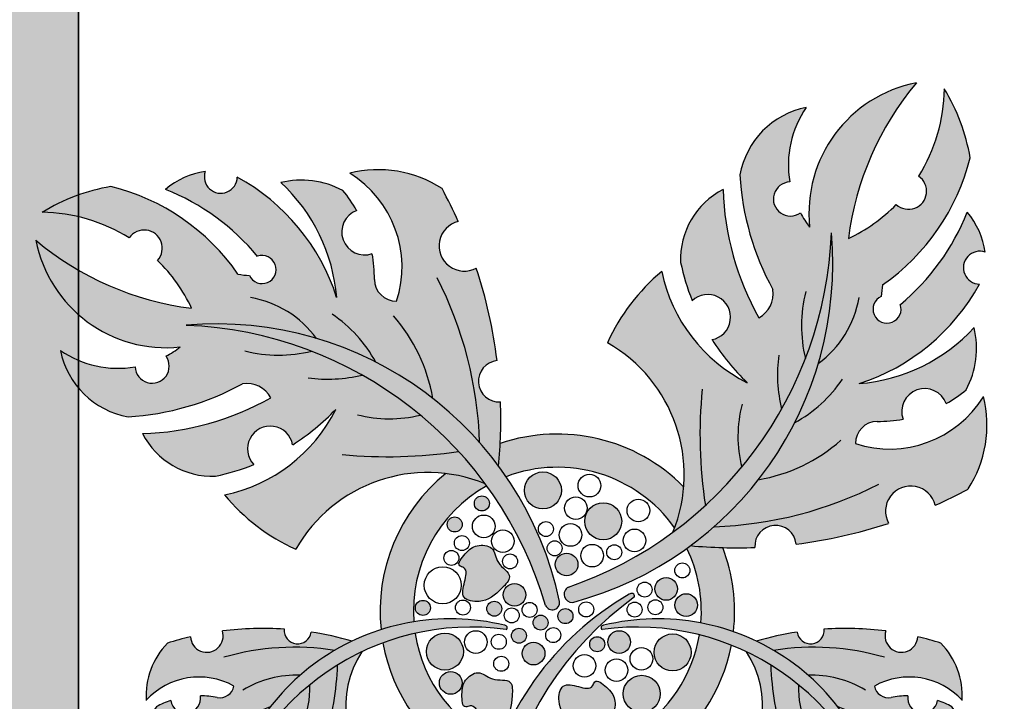
# Model space of a CAD drawing. Units: inches. Extents: x 3008 to 4088, y 1255 to 2137.
# Tile 15 of 30: x 3042 to 3093, y 1874 to 1909. Entities that reach past the tile are written whole.
import ezdxf

# ---------------------------------------------------------------- set-up
doc = ezdxf.new("R2010")
doc.units = ezdxf.units.IN
for name, color, linetype, lineweight in [('C-PROP', 1, 'Continuous', 35), ('C-PROP-PATT', 9, 'Continuous', 13), ('estofado', 7, 'Continuous', 25), ('L-PLNT', 3, 'Continuous', 13)]:
    doc.layers.add(name, color=color, linetype=linetype, lineweight=lineweight)

# ---------------------------------------------------------------- blocks, each defined once
blk = doc.blocks.new('Novo Cashepo')
at = {"layer": 'estofado', "ltscale": 0.1}
h = blk.add_hatch(color=256, dxfattribs=at)
h.set_gradient(color1=(108, 164, 86), color2=(79, 120, 63), one_color=1, tint=0.36, name='CYLINDER')
h.paths.add_polyline_path([(0.2827, 0.4266, -0.314907), (0.2643, 0.3891, -0.122145), (0.2167, 0.5593, 0.291545), (0.1604, 0.4626, 0.043027), (0.1756, 0.4118, -1.339402), (0.202, 0.3602, 0.060072), (0.2488, 0.3031, -0.231117), (0.1355, 0.4506, 0.11449), (0.0635, 0.3561, -0.376746), (0.1502, 0.1049, 0.228124), (0.3602, 0.5016, -0.2613), (0.1736, 0.0872, 0.033062), (0.2588, 0.0848, -0.981895), (0.3134, 0.0893, 0.048855), (0.4361, 0.1168, -1.138233), (0.4978, 0.1407, 0.018864), (0.5414, 0.1623, 0.208979), (0.5618, 0.2847, -0.346636), (0.3922, 0.2224, -0.42625), (0.4225, 0.2519, 0.04537), (0.4552, 0.2547, -0.994855), (0.5125, 0.2753, 0.044381), (0.539, 0.2936, 0.18118), (0.5496, 0.3761, -0.18833), (0.3972, 0.3019, 0.191426), (0.5567, 0.4338, -1.174476), (0.5643, 0.4761, 0.140528), (0.5404, 0.529, -0.125367), (0.4517, 0.4068, -2.245001), (0.4262, 0.4175, -0.031976), (0.4282, 0.4328, 0.181425), (0.5443, 0.6013, 0.094503), (0.51, 0.6925, -0.138196), (0.476, 0.5769, -1.074478), (0.4463, 0.5393, -0.088291), (0.3828, 0.4942, -0.144087), (0.473, 0.7006, 0.388768), (0.3315, 0.5094, -0.041945), (0.3192, 0.5282, -1.340573), (0.3051, 0.5692, -0.196063), (0.327, 0.668, 0.307628), (0.2389, 0.5784, 0.111291)])
h = blk.add_hatch(color=256, dxfattribs=at)
h.set_gradient(color1=(108, 164, 86), color2=(102, 154, 81), one_color=1, tint=0.46, name='CYLINDER')
h.paths.add_polyline_path([(-0.0809, 0.1926, 0.033062), (-0.0785, 0.2778, -0.981895), (-0.0829, 0.3324, 0.048855), (-0.1105, 0.4551, -1.138233), (-0.1344, 0.5168, 0.018864), (-0.1559, 0.5604, 0.208979), (-0.2783, 0.5808, -0.346636), (-0.2161, 0.4112, -0.42625), (-0.2455, 0.4415, 0.04537), (-0.2484, 0.4742, -0.994855), (-0.269, 0.5315, 0.044381), (-0.2872, 0.5579, 0.18118), (-0.3697, 0.5686, -0.18833), (-0.2956, 0.4161, 0.191426), (-0.4275, 0.5757, -1.174476), (-0.4698, 0.5832, 0.140528), (-0.5227, 0.5593, -0.125367), (-0.4005, 0.4706, -2.245001), (-0.4112, 0.4452, -0.031976), (-0.4264, 0.4471, 0.181425), (-0.595, 0.5633, 0.094503), (-0.6862, 0.529, -0.138196), (-0.5706, 0.495, -1.074478), (-0.5329, 0.4652, -0.088291), (-0.4878, 0.4018, -0.144087), (-0.6943, 0.4919, 0.388768), (-0.503, 0.3504, -0.041945), (-0.5218, 0.3381, -1.340573), (-0.5628, 0.324, -0.196063), (-0.6617, 0.346, 0.307628), (-0.5721, 0.2579, 0.111291), (-0.4203, 0.3017, -0.314907), (-0.3828, 0.2833, -0.122145), (-0.553, 0.2356, 0.291545), (-0.4562, 0.1793, 0.043027), (-0.4055, 0.1946, -1.339402), (-0.3539, 0.2209, 0.060072), (-0.2968, 0.2677, -0.231117), (-0.4442, 0.1544, 0.11449), (-0.3498, 0.0824, -0.376746), (-0.0985, 0.1691, 0.228124), (-0.4952, 0.3792, -0.2613)])
h = blk.add_hatch(color=256, dxfattribs=at)
h.set_gradient(color1=(166, 115, 84), color2=(109, 75, 55), one_color=1, tint=0.32, name='INVCYLINDER')
h.paths.add_polyline_path([(0.3602, 0.5016, -0.309503), (0.0116, 0.0322, 0.812635), (0.0173, 0.012, 0.364481)])
h = blk.add_hatch(color=256, dxfattribs=at)
h.set_gradient(color1=(166, 115, 84), color2=(109, 75, 55), one_color=1, tint=0.32, name='INVCYLINDER')
h.paths.add_polyline_path([(-0.0186, 0.0079, 0.872708), (-0.0001, 0.0132, 0.378997), (-0.4952, 0.3792, -0.322151)])
h = blk.add_hatch(color=256, dxfattribs=at)
h.set_gradient(color1=(185, 193, 193), color2=(81, 92, 92), one_color=1, tint=0.34, name='CURVED')
h.paths.add_polyline_path([(0.1525, 0.1108, 0.06904), (0.1645, 0.1649, 0.288006), (-0.0787, 0.2226, -0.011646), (-0.0809, 0.1926, -0.009266), (-0.0709, 0.1786, -0.341204)])
h = blk.add_hatch(color=256, dxfattribs=at)
h.set_gradient(color1=(179, 165, 128), color2=(150, 134, 90), one_color=1, tint=0.47)
h.paths.add_polyline_path([(-0.0466, 0.1604, -1), (0.0024, 0.1604, -1)])
h = blk.add_hatch(color=256, dxfattribs=at)
h.set_gradient(color1=(185, 193, 193), color2=(81, 92, 92), one_color=1, tint=0.34, name='CURVED')
h.paths.add_polyline_path([(-0.0966, 0.1665, 0.00155), (-0.0985, 0.1691, 0.067559), (-0.151, 0.1827, 0.253608), (-0.2368, -0.0242, -0.036817), (-0.1935, -0.0138, -0.290631)])
h = blk.add_hatch(color=256, dxfattribs=at)
h.set_gradient(color1=(179, 165, 128), color2=(150, 134, 90), one_color=1, tint=0.47)
h.paths.add_polyline_path([(-0.113, 0.1431, 1), (-0.0932, 0.1431, 1)])
h = blk.add_hatch(color=256, dxfattribs=at)
h.set_gradient(color1=(179, 165, 128), color2=(150, 134, 90), one_color=1, tint=0.47)
h.paths.add_polyline_path([(0.0333, 0.1194, 1), (0.0824, 0.1194, 1)])
h = blk.add_hatch(color=256, dxfattribs=at)
h.set_gradient(color1=(179, 165, 128), color2=(150, 134, 90), one_color=1, tint=0.47)
h.paths.add_polyline_path([(-0.149, 0.1152, 1), (-0.1291, 0.1152, 1)])
h = blk.add_hatch(color=256, dxfattribs=at)
h.set_gradient(color1=(179, 165, 128), color2=(150, 134, 90), one_color=1, tint=0.47)
edge = h.paths.add_edge_path()
edge.add_spline(control_points=[(-0.126, 0.0391), (-0.128, 0.0314), (-0.132, 0.0156), (-0.099, 0.0101), (-0.0817, 0.025), (-0.0594, 0.0483), (-0.0851, 0.062), (-0.0856, 0.0869), (-0.1113, 0.0892), (-0.1235, 0.079), (-0.1379, 0.0613), (-0.1214, 0.0568), (-0.124, 0.0467), (-0.126, 0.0391)], knot_values=[0, 0, 0, 0, 0.020201, 0.040881, 0.075874, 0.093984, 0.117931, 0.138882, 0.158108, 0.177537, 0.194687, 0.200618, 0.219249, 0.219249, 0.219249, 0.219249], degree=3, periodic=0)
h = blk.add_hatch(color=256, dxfattribs=at)
h.set_gradient(color1=(185, 193, 193), color2=(81, 92, 92), one_color=1, tint=0.34, name='CURVED')
h.paths.add_polyline_path([(0.1736, 0.0872, -0.003321), (0.1687, 0.0836, -0.134103), (0.1873, -0.0153, -0.036923), (0.2304, -0.0269, 0.121396), (0.2162, 0.0846, -0.016535)])
h = blk.add_hatch(color=256, dxfattribs=at)
h.set_gradient(color1=(179, 165, 128), color2=(150, 134, 90), one_color=1, tint=0.47)
h.paths.add_polyline_path([(0.0244, 0.0622, 1), (-0.0057, 0.0622, 1)])
h = blk.add_hatch(color=256, dxfattribs=at)
h.set_gradient(color1=(179, 165, 128), color2=(150, 134, 90), one_color=1, tint=0.47)
h.paths.add_polyline_path([(0.1562, 0.0298, 1), (0.1262, 0.0298, 1)])
h = blk.add_hatch(color=256, dxfattribs=at)
h.set_gradient(color1=(179, 165, 128), color2=(150, 134, 90), one_color=1, tint=0.47)
h.paths.add_polyline_path([(-0.0448, 0.022, 1), (-0.0748, 0.022, 1)])
h = blk.add_hatch(color=256, dxfattribs=at)
h.set_gradient(color1=(179, 165, 128), color2=(150, 134, 90), one_color=1, tint=0.47)
h.paths.add_polyline_path([(-0.1713, 0.0047, 1), (-0.1912, 0.0047, 1)])
h = blk.add_hatch(color=256, dxfattribs=at)
h.set_gradient(color1=(166, 115, 84), color2=(109, 75, 55), one_color=1, tint=0.32, name='INVCYLINDER')
h.paths.add_polyline_path([(0.0994, 0.0192, 0.726279), (0.0923, 0.0227, 0.000011), (0.0923, 0.0227, 0.454782), (-0.024, -0.5707, -0.387777)])
h = blk.add_hatch(color=256, dxfattribs=at)
h.set_gradient(color1=(179, 165, 128), color2=(150, 134, 90), one_color=1, tint=0.47)
h.paths.add_polyline_path([(-0.0766, 0.0036, 1), (-0.0965, 0.0036, 1)])
h = blk.add_hatch(color=256, dxfattribs=at)
h.set_gradient(color1=(179, 165, 128), color2=(150, 134, 90), one_color=1, tint=0.47)
h.paths.add_polyline_path([(0.1828, 0.0084, 1), (0.1527, 0.0084, 1)])
h = blk.add_hatch(color=256, dxfattribs=at)
h.set_gradient(color1=(179, 165, 128), color2=(150, 134, 90), one_color=1, tint=0.47)
h.paths.add_polyline_path([(0.0176, -0.0063, 1), (-0.0023, -0.0063, 1)])
h = blk.add_hatch(color=256, dxfattribs=at)
h.set_gradient(color1=(166, 115, 84), color2=(109, 75, 55), one_color=1, tint=0.32, name='INVCYLINDER')
h.paths.add_polyline_path([(-0.0708, -0.0241, 0.529291), (-0.0712, -0.0189, 0.456534), (-0.4459, -0.2817, -0.387777)])
h = blk.add_hatch(color=256, dxfattribs=at)
h.set_gradient(color1=(179, 165, 128), color2=(150, 134, 90), one_color=1, tint=0.47)
h.paths.add_polyline_path([(-0.0152, -0.0149, 1), (-0.0351, -0.0149, 1)])
h = blk.add_hatch(color=256, dxfattribs=at)
h.set_gradient(color1=(166, 115, 84), color2=(109, 75, 55), one_color=1, tint=0.32, name='INVCYLINDER')
h.paths.add_polyline_path([(0.4314, -0.2817, 0.456534), (0.0566, -0.0189, 0.529291), (0.0563, -0.0241, -0.387777)])
h = blk.add_hatch(color=256, dxfattribs=at)
h.set_gradient(color1=(108, 164, 86), color2=(62, 94, 49), one_color=1, tint=0.28, name='CURVED')
h.paths.add_polyline_path([(-0.5633, -0.214, -1.174476), (-0.5734, -0.2402, 0.140528), (-0.5646, -0.277, -0.125367), (-0.4927, -0.2097, -2.245001), (-0.4777, -0.2197, -0.031976), (-0.4809, -0.2292, 0.181425), (-0.5761, -0.3228, 0.094503), (-0.5654, -0.3855, -0.138196), (-0.5293, -0.3156, -1.074478), (-0.5056, -0.2952, -0.088291), (-0.4594, -0.2742, -0.144087), (-0.5427, -0.3952, 0.388768), (-0.4284, -0.2902, -0.041945), (-0.4229, -0.3038, -1.340573), (-0.4189, -0.3318, -0.196063), (-0.4452, -0.3924, 0.307628), (-0.3777, -0.3459, 0.111291), (-0.387, -0.2433, -0.314907), (-0.3706, -0.2216, -0.122145), (-0.3611, -0.3364, 0.291545), (-0.3131, -0.2814, 0.043027), (-0.3166, -0.247, -1.339402), (-0.3271, -0.2108, 0.060072), (-0.35, -0.1684, -0.231117), (-0.2957, -0.2768, 0.11449), (-0.2379, -0.2252, -0.376746), (-0.2623, -0.0537, 0.228124), (-0.4459, -0.2817, -0.2613), (-0.2752, -0.0394, 0.033062), (-0.3295, -0.0274, -0.981895), (-0.365, -0.0235, 0.048855), (-0.4469, -0.026, -1.138233), (-0.4894, -0.0336, 0.018864), (-0.52, -0.042, 0.208979), (-0.5481, -0.1179, -0.346636), (-0.4319, -0.099, -0.42625), (-0.4549, -0.1141, 0.04537), (-0.4762, -0.1119, -0.994855), (-0.5154, -0.118, 0.044381), (-0.5346, -0.1264, 0.18118), (-0.5516, -0.1779, -0.18833), (-0.4449, -0.1493, 0.191426)])
h = blk.add_hatch(color=256, dxfattribs=at)
h.set_gradient(color1=(179, 165, 128), color2=(150, 134, 90), one_color=1, tint=0.47)
h.paths.add_polyline_path([(-0.0439, -0.0322, 1), (-0.0638, -0.0322, 1)])
h = blk.add_hatch(color=256, dxfattribs=at)
h.set_gradient(color1=(179, 165, 128), color2=(150, 134, 90), one_color=1, tint=0.47)
h.paths.add_polyline_path([(0.0939, -0.0406, 1), (0.0639, -0.0406, 1)])
h = blk.add_hatch(color=256, dxfattribs=at)
h.set_gradient(color1=(108, 164, 86), color2=(154, 193, 138), one_color=1, tint=0.65, name='HEMISPHERICAL')
h.paths.add_polyline_path([(0.4174, -0.099, -0.346636), (0.5336, -0.1179, 0.208979), (0.5055, -0.042, 0.018864), (0.4749, -0.0336, -1.138233), (0.4324, -0.026, 0.048855), (0.3504, -0.0235, -0.981895), (0.3149, -0.0274, 0.033062), (0.2607, -0.0394, -0.2613), (0.4314, -0.2817, 0.228124), (0.2478, -0.0537, -0.376746), (0.2234, -0.2252, 0.11449), (0.2812, -0.2768, -0.231117), (0.3355, -0.1684, 0.060072), (0.3126, -0.2108, -1.339402), (0.3021, -0.247, 0.043027), (0.2986, -0.2814, 0.291545), (0.3466, -0.3364, -0.122145), (0.3561, -0.2216, -0.314907), (0.3725, -0.2433, 0.111291), (0.3632, -0.3459, 0.307628), (0.4307, -0.3924, -0.196063), (0.4044, -0.3318, -1.340573), (0.4084, -0.3038, -0.041945), (0.4139, -0.2902, 0.388768), (0.5282, -0.3952, -0.144087), (0.4449, -0.2742, -0.088291), (0.4911, -0.2952, -1.074478), (0.5148, -0.3156, -0.138196), (0.5509, -0.3855, 0.094503), (0.5616, -0.3228, 0.181425), (0.4664, -0.2292, -0.031976), (0.4632, -0.2197, -2.245001), (0.4782, -0.2097, -0.125367), (0.5501, -0.277, 0.140528), (0.5589, -0.2402, -1.174476), (0.5488, -0.214, 0.191426), (0.4304, -0.1493, -0.18833), (0.5371, -0.1779, 0.18118), (0.5201, -0.1264, 0.044381), (0.5009, -0.118, -0.994855), (0.4617, -0.1119, 0.04537), (0.4404, -0.1141, -0.42625)])
h = blk.add_hatch(color=256, dxfattribs=at)
h.set_gradient(color1=(185, 193, 193), color2=(81, 92, 92), one_color=1, tint=0.34, name='CURVED')
h.paths.add_polyline_path([(-0.1917, -0.0292, 0.03292), (-0.2343, -0.0418, 0.221446), (-0.1198, -0.2039, -0.019377), (-0.0822, -0.1825, -0.005069), (-0.0793, -0.175, -0.256969)])
h = blk.add_hatch(color=256, dxfattribs=at)
h.set_gradient(color1=(179, 165, 128), color2=(150, 134, 90), one_color=1, tint=0.47)
h.paths.add_polyline_path([(-0.1275, -0.0533, 1), (-0.1765, -0.0533, 1)])
h = blk.add_hatch(color=256, dxfattribs=at)
h.set_gradient(color1=(185, 193, 193), color2=(81, 92, 92), one_color=1, tint=0.34, name='CURVED')
h.paths.add_polyline_path([(0.1853, -0.0311, -0.449638), (-0.0565, -0.1832, 0.000699), (-0.0569, -0.1844, 0.072477), (-0.0408, -0.2319, 0.40511), (0.2276, -0.0448, 0.032975)])
h = blk.add_hatch(color=256, dxfattribs=at)
h.set_gradient(color1=(179, 165, 128), color2=(150, 134, 90), one_color=1, tint=0.47)
h.paths.add_polyline_path([(0.0597, -0.0435, 1), (0.0398, -0.0435, 1)])
h = blk.add_hatch(color=256, dxfattribs=at)
h.set_gradient(color1=(179, 165, 128), color2=(150, 134, 90), one_color=1, tint=0.47)
h.paths.add_polyline_path([(0.1743, -0.0543, 1), (0.1253, -0.0543, 1)])
h = blk.add_hatch(color=256, dxfattribs=at)
h.set_gradient(color1=(179, 165, 128), color2=(150, 134, 90), one_color=1, tint=0.47)
h.paths.add_polyline_path([(-0.0194, -0.0559, 1), (-0.0495, -0.0559, 1)])
h = blk.add_hatch(color=256, dxfattribs=at)
h.set_gradient(color1=(179, 165, 128), color2=(150, 134, 90), one_color=1, tint=0.47)
edge = h.paths.add_edge_path()
edge.add_spline(control_points=[(-0.1055, -0.1384), (-0.1019, -0.1456), (-0.0945, -0.16), (-0.0661, -0.1423), (-0.063, -0.1197), (-0.0617, -0.0875), (-0.09, -0.0942), (-0.1068, -0.0758), (-0.1276, -0.0911), (-0.13, -0.1069), (-0.1291, -0.1297), (-0.1137, -0.1221), (-0.1091, -0.1314), (-0.1055, -0.1384)], knot_values=[0, 0, 0, 0, 0.020201, 0.040881, 0.075874, 0.093984, 0.117931, 0.138882, 0.158108, 0.177537, 0.194687, 0.200618, 0.219249, 0.219249, 0.219249, 0.219249], degree=3, periodic=0)
h = blk.add_hatch(color=256, dxfattribs=at)
h.set_gradient(color1=(179, 165, 128), color2=(150, 134, 90), one_color=1, tint=0.47)
h.paths.add_polyline_path([(-0.1294, -0.0948, 1), (-0.1594, -0.0948, 1)])
h = blk.add_hatch(color=256, dxfattribs=at)
h.set_gradient(color1=(179, 165, 128), color2=(150, 134, 90), one_color=1, tint=0.47)
edge = h.paths.add_edge_path()
edge.add_spline(control_points=[(0.0251, -0.0997), (0.0173, -0.0977), (0.0016, -0.0937), (-0.004, -0.1268), (0.011, -0.1441), (0.0343, -0.1664), (0.0479, -0.1407), (0.0728, -0.1402), (0.0751, -0.1145), (0.0649, -0.1023), (0.0473, -0.0879), (0.0427, -0.1044), (0.0327, -0.1017), (0.0251, -0.0997)], knot_values=[0, 0, 0, 0, 0.020201, 0.040881, 0.075874, 0.093984, 0.117931, 0.138882, 0.158108, 0.177537, 0.194687, 0.200618, 0.219249, 0.219249, 0.219249, 0.219249], degree=3, periodic=0)
h = blk.add_hatch(color=256, dxfattribs=at)
h.set_gradient(color1=(179, 165, 128), color2=(150, 134, 90), one_color=1, tint=0.47)
h.paths.add_polyline_path([(0.1333, -0.1092, 1), (0.0843, -0.1092, 1)])
h = blk.add_hatch(color=256, dxfattribs=at)
h.set_gradient(color1=(108, 164, 86), color2=(128, 178, 108), one_color=1, tint=0.56, name='CYLINDER')
h.paths.add_polyline_path([(-0.0931, -0.2153, -0.021499), (-0.0822, -0.1825, 0.033062), (-0.1452, -0.2207, -0.981895), (-0.1828, -0.2494, 0.048855), (-0.259, -0.3268, -1.138233), (-0.2927, -0.373, 0.018864), (-0.3143, -0.409, 0.208979), (-0.2718, -0.5074, -0.346636), (-0.1778, -0.383, -0.218356), (-0.1066, -0.288, -0.045186), (-0.0935, -0.2168, -0.00127), (-0.0946, -0.2163, -0.001036)])
h = blk.add_hatch(color=256, dxfattribs=at)
h.set_gradient(color1=(108, 164, 86), color2=(128, 178, 108), one_color=1, tint=0.56, name='CYLINDER')
h.paths.add_polyline_path([(0.1153, -0.4286, 0.11449), (0.1235, -0.3263, -0.376746), (-0.0569, -0.1844, 0.228124), (-0.024, -0.5707, -0.289779), (-0.0128, -0.768, 0.388768), (0.0005, -0.5629, -0.041945), (0.0182, -0.5708, -1.340573), (0.0477, -0.594, -0.196063), (0.0779, -0.676, 0.307628), (0.1, -0.5698, 0.111291), (-0.0028, -0.48, -0.314907), (-0.0069, -0.4442, -0.122145), (0.1072, -0.5455, 0.291545), (0.1029, -0.4489, 0.043027), (0.0681, -0.4192, -1.339402), (0.0248, -0.3941, 0.060072), (-0.0358, -0.3745, -0.231117)])
h = blk.add_hatch(color=256, dxfattribs=at)
h.set_gradient(color1=(108, 164, 86), color2=(128, 178, 108), one_color=1, tint=0.56, name='CYLINDER')
h.paths.add_polyline_path([(-0.186, -0.4185, 0.04537), (-0.2084, -0.4358, -0.994855), (-0.2404, -0.4776, 0.044381), (-0.2511, -0.5032, 0.18118), (-0.2202, -0.5681, -0.18833), (-0.1442, -0.443, 0.191426), (-0.1984, -0.6134, -0.461932), (-0.1711, -0.6221, -0.164855), (-0.099, -0.4106, -0.076989), (-0.1066, -0.288, 0.218356), (-0.1778, -0.383, -0.42625)])
h = blk.add_hatch(color=256, dxfattribs=at)
h.set_gradient(color1=(108, 164, 86), color2=(128, 178, 108), one_color=1, tint=0.56, name='CYLINDER')
h.paths.add_polyline_path([(-0.1111, -0.7292, 0.094503), (-0.0435, -0.7794, -0.138196), (-0.0729, -0.6796, -1.074478), (-0.0689, -0.6383, -0.088291), (-0.0439, -0.5759, -0.144087), (-0.0128, -0.768, 0.289779), (-0.024, -0.5707, -0.111568), (-0.099, -0.4106, 0.164855), (-0.1711, -0.6221, -0.461932), (-0.1841, -0.6476, 0.140528), (-0.142, -0.6749, -0.125367), (-0.1347, -0.5446, -2.245001), (-0.1112, -0.5405, -0.031976), (-0.1055, -0.5525, 0.181425)])
for centre, radius in [((-0.0221, 0.1604), 0.0245), ((0.0395, 0.1667), 0.015), ((-0.1031, 0.1431), 0.00994), ((0.0215, 0.1368), 0.015), ((0.0578, 0.1194), 0.0245), ((0.1044, 0.1338), 0.015), ((-0.1391, 0.1152), 0.00994), ((-0.1006, 0.1127), 0.015), ((-0.0182, 0.1092), 0.00994), ((-0.0753, 0.0931), 0.015), ((0.0145, 0.1013), 0.015), ((0.0993, 0.0941), 0.015), ((-0.1296, 0.0906), 0.00994), ((-0.0066, 0.0836), 0.00994), ((-0.1435, 0.0709), 0.00994), ((0.0432, 0.0739), 0.015), ((0.0724, 0.0784), 0.00994), ((-0.0657, 0.0663), 0.00994), ((0.0093, 0.0622), 0.015), ((-0.155, 0.0346), 0.0245), ((0.1627, 0.0543), 0.00994), ((0.1412, 0.0298), 0.015), ((-0.0598, 0.022), 0.015), ((0.1127, 0.0289), 0.00994), ((-0.1813, 0.0047), 0.00994), ((-0.1282, 0.0051), 0.00994), ((-0.0866, 0.0036), 0.00994), ((0.127, 0.0055), 0.00994), ((0.1678, 0.0084), 0.015), ((-0.0635, -0.0053), 0.00994), ((-0.0398, 0.002), 0.00994), ((0.0077, -0.0063), 0.00994), ((0.0352, 0.0026), 0.00994), ((0.0994, 0.0024), 0.00994), ((-0.0252, -0.0149), 0.00994), ((-0.1111, -0.0406), 0.015), ((-0.0539, -0.0322), 0.00994), ((-0.0085, -0.0314), 0.00994), ((0.0789, -0.0406), 0.015), ((-0.152, -0.0533), 0.0245), ((-0.0806, -0.0403), 0.00994), ((0.0498, -0.0435), 0.00994), ((0.1498, -0.0543), 0.0245), ((-0.0345, -0.0559), 0.015), ((0.1084, -0.0629), 0.015), ((-0.0774, -0.0694), 0.00994), ((0.0329, -0.0722), 0.015), ((0.0754, -0.0779), 0.015), ((-0.1444, -0.0948), 0.015), ((0.1088, -0.1092), 0.0245), ((-0.0125, -0.1547), 0.015), ((0.0867, -0.1514), 0.00994), ((0.0538, -0.1663), 0.00994)]:
    blk.add_circle(centre, radius, dxfattribs=at)
for centre, radius, start, end in [((0.5066, 0.5278), 0.1761, 101.0186, 185.9966), ((0.7787, 0.4442), 0.399, 140.0122, 172.8088), ((0.2879, 0.6951), 0.2222, 327.8752, 359.3481), ((0.2881, 0.557), 0.26, 9.8207, 31.4151), ((0.3489, 0.5584), 0.1118, 101.2825, 169.6799), ((0.4372, 0.5917), 0.134, 145.305, 189.6765), ((0.2616, 0.6719), 0.2914, 304.8613, 345.9935), ((-0.4545, 0.479), 0.1053, 98.3059, 130.3029), ((-0.4492, 0.576), 0.0218, 160.6631, 359.0131), ((-0.5622, 0.33), 0.2802, 17.9062, 61.2534), ((-0.2404, 0.4305), 0.1549, 56.9429, 104.1578), ((-0.3548, 0.4565), 0.1459, 341.9118, 58.3844), ((0.5976, 0.5997), 0.3593, 183.393, 208.7944), ((0.4625, 0.557), 0.024, 227.5673, 55.7919), ((-0.5506, 0.307), 0.26, 99.8207, 121.4151), ((-0.6655, 0.2806), 0.2914, 34.8613, 75.9935), ((-0.3427, 0.4531), 0.1185, 62.1153, 103.1932), ((-0.5278, 0.3974), 0.233, 4.6076, 47.2701), ((0.306, 0.5466), 0.0226, 92.4292, 305.5449), ((-0.6357, 0.2751), 0.3059, 39.7257, 68.3087), ((-0.4269, 0.4422), 0.1813, 29.481, 39.6456), ((-0.7231, 0.2531), 0.6451, 24.1234, 28.4463), ((0.2645, 0.4667), 0.1042, 117.2921, 182.3073), ((0.5836, 0.5703), 0.3671, 181.7055, 209.5612), ((0.2879, 0.6951), 0.2222, 295.3016, 315.484), ((-0.6887, 0.3068), 0.2222, 57.8752, 89.3481), ((-0.2585, 0.5029), 0.0304, 110.1108, 289.5198), ((0.4372, 0.5917), 0.134, 208.2976, 217.9049), ((0.2562, 0.6421), 0.3059, 309.7257, 338.3087), ((0.4601, 0.4609), 0.1053, 8.3059, 40.3029), ((-0.1264, 0.4844), 0.0334, 103.7865, 298.5822), ((-0.5507, 0.4815), 0.024, 317.5673, 145.7919), ((-0.1569, 0.5215), 0.5175, 289.0066, 357.7964), ((-0.1024, 0.4607), 0.4645, 284.942, 5.0453), ((-0.4379, 0.7976), 0.399, 230.0122, 262.8088), ((-0.5214, 0.5256), 0.1761, 191.0186, 275.9966), ((-0.3944, 0.4531), 0.0186, 205.201, 109.1617), ((-0.4269, 0.4422), 0.1813, 359.2754, 10.1496), ((0.5571, 0.4556), 0.0218, 70.6631, 269.0131), ((-0.6887, 0.3068), 0.2222, 25.3016, 45.484), ((0.4622, 0.5257), 0.3083, 191.8137, 201.6687), ((-0.4035, 0.5652), 0.1203, 259.0186, 266.3445), ((-0.7231, 0.2531), 0.6451, 7.0576, 18.2453), ((0.303, 0.2481), 0.2627, 129.608, 155.7334), ((0.3431, 0.4928), 0.2118, 191.5061, 243.5602), ((-0.2163, 0.4404), 0.0293, 181.0153, 270.3634), ((-0.6263, 0.2061), 0.5206, 1.9256, 26.9542), ((0.311, 0.5686), 0.2802, 287.9062, 331.2534), ((0.5463, 0.4099), 0.1203, 169.0186, 176.3445), ((0.1964, 0.3899), 0.0302, 280.5489, 133.5686), ((0.2467, 0.421), 0.0364, 298.8789, 8.7972), ((0.5076, 0.3784), 0.1869, 165.9423, 193.4167), ((-0.4326, 0.2811), 0.1367, 36.1411, 80.3873), ((0.2622, 0.4389), 0.1367, 306.1411, 350.3873), ((0.4341, 0.4007), 0.0186, 115.201, 19.1617), ((-0.4031, 0.2432), 0.1817, 28.6905, 56.0246), ((-0.3847, 0.2462), 0.2195, 9.4944, 41.5537), ((-0.4544, -0.0835), 0.4645, 12.0191, 95.0453), ((-0.5151, -0.138), 0.5175, 16.3708, 87.7964), ((0.3785, 0.5342), 0.233, 274.6076, 317.2701), ((0.4342, 0.349), 0.1185, 332.1153, 13.1932), ((-0.0362, 0.1811), 0.2014, 337.7465, 60.3213), ((0.4622, 0.5257), 0.3083, 212.4488, 226.1997), ((-0.5854, 0.4562), 0.134, 235.305, 279.6765), ((-0.5521, 0.3678), 0.1118, 191.2825, 259.6799), ((-0.5854, 0.4562), 0.134, 298.2976, 307.9049), ((-0.372, 0.5266), 0.1869, 255.9423, 283.4167), ((0.4824, 0.3139), 0.1936, 172.3137, 193.7119), ((-0.5402, 0.325), 0.0226, 182.4292, 35.5449), ((-0.0802, 0.3051), 0.0274, 95.6708, 273.5772), ((-0.5933, 0.6166), 0.3593, 273.393, 298.7944), ((-0.4147, 0.2657), 0.0364, 28.8789, 98.7972), ((-0.3076, 0.5014), 0.1936, 262.3137, 283.7119), ((0.2242, 0.4094), 0.1817, 298.6905, 326.0246), ((0.8078, 0.234), 0.6217, 174.4084, 188.6615), ((0.4839, 0.2649), 0.0304, 20.1108, 199.5198), ((0.4233, 0.4332), 0.1813, 299.481, 309.6456), ((-0.5639, 0.6026), 0.3671, 271.7055, 299.5612), ((-0.7231, 0.2531), 0.6451, 354.6159, 2.1904), ((0.4075, 0.2318), 0.1711, 165.544, 193.8081), ((0.4375, 0.3611), 0.1459, 251.9118, 328.3844), ((0.4116, 0.2468), 0.1549, 326.9429, 14.1578), ((-0.4865, 0.362), 0.2118, 281.5061, 333.5602), ((-0.5193, 0.4811), 0.3083, 302.4488, 316.1997), ((-0.2254, 0.4264), 0.1711, 255.544, 283.8081), ((0.4215, 0.2226), 0.0293, 91.0153, 180.3634), ((0.4233, 0.4332), 0.1813, 269.2754, 280.1496), ((-0.4604, 0.2834), 0.1042, 207.2921, 272.3073), ((-0.3836, 0.2154), 0.0302, 10.5489, 223.5686), ((-0.003, 0.0001), 0.235, 44.5248, 108.7916), ((0.2272, 0.3911), 0.2195, 279.4944, 311.5537), ((-0.2276, 0.8267), 0.6217, 264.4084, 278.6615), ((-0.5193, 0.4811), 0.3083, 281.8137, 291.6687), ((-0.1748, -0.0173), 0.2014, 67.7465, 150.3213), ((-0.003, 0.0001), 0.1909, 35.4554, 110.8148), ((-0.003, 0.0001), 0.235, 129.0122, 185.9347), ((-0.003, 0.0001), 0.1909, 119.3518, 184.1737), ((0.1872, 0.6326), 0.5206, 271.9256, 296.9542), ((0.4654, 0.1328), 0.0334, 13.7865, 208.5822), ((0.2342, 0.7294), 0.6451, 294.1234, 298.4463), ((-0.2418, 0.3219), 0.2627, 219.608, 245.7334), ((0.2862, 0.0866), 0.0274, 5.6708, 183.5772), ((0.2342, 0.7294), 0.6451, 277.0576, 288.2453), ((-0.003, 0.0001), 0.1909, 355.3819, 25.9338), ((0.2342, 0.7294), 0.6451, 264.6159, 272.1904), ((-0.003, 0.0001), 0.235, 353.3979, 21.0844), ((0.0166, 0.0227), 0.0107, 117.5535, 273.9476), ((0.2929, -0.3247), 0.4012, 120.0005, 217.8213), ((0.3609, -0.3433), 0.447, 125.7916, 210.5723), ((-0.0097, 0.0118), 0.00971, 203.8853, 8.3312), ((0.0953, 0.0198), 0.00417, 352.069, 136.0321), ((-0.1446, -0.3127), 0.3029, 76.2995, 174.1203), ((0.1301, -0.3127), 0.3029, 5.8797, 103.7005), ((-0.4677, -0.0325), 0.0217, 182.8615, 17.6572), ((-0.3933, -0.4432), 0.4207, 86.1325, 97.3203), ((-0.1172, -0.3583), 0.3375, 82.0906, 166.8713), ((-0.3472, -0.0251), 0.0179, 174.7458, 352.6522), ((-0.0727, -0.0216), 0.00315, 308.368, 92.3311), ((0.0582, -0.0216), 0.00315, 87.6689, 231.632), ((0.1027, -0.3583), 0.3375, 13.1287, 97.9094), ((0.3327, -0.0251), 0.0179, 187.3478, 5.2542), ((0.3788, -0.4432), 0.4207, 82.6797, 93.8675), ((0.4531, -0.0325), 0.0217, 162.3428, 357.1385), ((-0.3933, -0.4432), 0.4207, 103.1984, 107.5212), ((-0.3933, -0.4432), 0.4207, 73.6909, 81.2654), ((-0.003, 0.0001), 0.1909, 188.82, 246.4657), ((-0.003, 0.0001), 0.1909, 253.7485, 350.5904), ((0.3788, -0.4432), 0.4207, 98.7346, 106.3091), ((0.3788, -0.4432), 0.4207, 72.4788, 76.8016), ((-0.4473, -0.1122), 0.101, 136.0179, 183.2328), ((-0.3513, -0.387), 0.3395, 81.0006, 106.0292), ((-0.003, 0.0001), 0.235, 190.2712, 240.2168), ((-0.003, 0.0001), 0.235, 260.7676, 348.9809), ((0.3368, -0.387), 0.3395, 73.9708, 98.9994), ((0.4328, -0.1122), 0.101, 356.7672, 43.9821), ((-0.1524, -0.1255), 0.1313, 146.8215, 229.3963), ((0.1379, -0.1255), 0.1313, 310.6037, 33.1785), ((-0.6994, -0.055), 0.4054, 343.4834, 357.7365), ((0.6849, -0.055), 0.4054, 182.2635, 196.5166), ((-0.478, -0.1822), 0.0952, 60.9868, 137.4594), ((-0.3471, -0.2274), 0.1431, 88.5693, 120.6287), ((0.3325, -0.2274), 0.1431, 59.3713, 91.4307), ((0.4635, -0.1822), 0.0952, 42.5406, 119.0132), ((-0.4506, -0.0955), 0.0191, 260.0903, 349.4383), ((-0.4428, -0.1031), 0.1116, 334.6189, 2.8831), ((0.4283, -0.1031), 0.1116, 177.1169, 205.3811), ((0.4361, -0.0955), 0.0191, 190.5617, 279.9097), ((-0.4958, -0.1149), 0.0199, 189.1858, 8.5947), ((-0.4778, -0.2301), 0.1183, 78.3504, 89.2246), ((0.4633, -0.2301), 0.1183, 90.7754, 101.6496), ((0.4813, -0.1149), 0.0199, 171.4053, 350.8142), ((-0.4744, -0.1749), 0.0773, 141.1903, 182.2681), ((-0.4778, -0.2301), 0.1183, 108.5559, 118.7205), ((-0.3474, -0.2395), 0.1185, 107.7654, 135.0996), ((0.3329, -0.2395), 0.1185, 44.9004, 72.2346), ((0.4633, -0.2301), 0.1183, 61.2795, 71.4441), ((0.4599, -0.1749), 0.0773, 357.7319, 38.8097), ((-0.5009, -0.1464), 0.1263, 341.3887, 2.7869), ((0.4864, -0.1464), 0.1263, 177.2131, 198.6113), ((-0.4227, -0.3307), 0.1827, 96.9812, 140.3284), ((-0.4616, -0.3003), 0.1519, 83.6826, 126.345), ((0.4471, -0.3003), 0.1519, 53.655, 96.3174), ((0.4082, -0.3307), 0.1827, 39.6716, 83.0188), ((-0.5141, -0.2845), 0.2011, 21.5237, 35.2746), ((-0.4338, -0.2782), 0.1381, 0.581, 52.6352), ((0.4193, -0.2782), 0.1381, 127.3648, 179.419), ((0.4996, -0.2845), 0.2011, 144.7254, 158.4763), ((-0.3754, -0.2537), 0.0892, 115.216, 159.4623), ((-0.525, -0.1846), 0.1219, 335.0173, 2.4916), ((0.1741, -0.6772), 0.5572, 117.3918, 124.9664), ((0.5105, -0.1846), 0.1219, 177.5084, 204.9827), ((0.3608, -0.2537), 0.0892, 20.5377, 64.784), ((0.1141, -0.1526), 0.1739, 190.5225, 273.0973), ((-0.4807, -0.208), 0.0121, 284.2759, 188.2367), ((0.4662, -0.208), 0.0121, 351.7633, 255.7241), ((-0.5662, -0.2279), 0.0142, 239.7381, 78.088), ((-0.3966, -0.3845), 0.1995, 118.8007, 147.3836), ((-0.5537, -0.2), 0.0785, 338.0936, 345.4195), ((-0.3633, -0.2442), 0.0238, 107.9539, 177.8722), ((-0.5974, -0.2981), 0.2394, 350.7805, 18.6362), ((-0.3272, -0.2305), 0.0197, 89.6239, 302.6435), ((0.1629, -0.585), 0.4497, 124.7016, 149.7302), ((-0.1643, -0.2347), 0.0237, 218.4468, 36.3532), ((-0.003, 0.0001), 0.235, 247.0716, 247.3627), ((0.3127, -0.2305), 0.0197, 237.3565, 90.3761), ((0.5829, -0.2981), 0.2394, 161.3638, 189.2195), ((0.3487, -0.2442), 0.0238, 2.1278, 72.0461), ((0.5392, -0.2), 0.0785, 194.5805, 201.9064), ((0.3821, -0.3845), 0.1995, 32.6164, 61.1993), ((0.5517, -0.2279), 0.0142, 101.912, 300.2619), ((-0.4038, -0.4029), 0.19, 113.9363, 155.0685), ((-0.3779, -0.1265), 0.1713, 298.683, 324.8084), ((-0.4741, -0.5856), 0.5369, 27.1843, 41.4375), ((0.3634, -0.1265), 0.1713, 215.1916, 241.317), ((0.3893, -0.4029), 0.19, 24.9315, 66.0637), ((-0.5048, -0.2433), 0.0687, 177.3808, 209.3779), ((-0.61, -0.3152), 0.2343, 352.4679, 17.8694), ((-0.5141, -0.2845), 0.2011, 0.8887, 10.7437), ((0.4996, -0.2845), 0.2011, 169.2563, 179.1113), ((0.5955, -0.3152), 0.2343, 162.1306, 187.5321), ((0.4903, -0.2433), 0.0687, 330.6221, 2.6192), ((0.1741, -0.6772), 0.5572, 129.8335, 141.0213), ((-0.7067, -0.1933), 0.2602, 309.0872, 341.8838), ((-0.4235, -0.4145), 0.1449, 104.3766, 124.559), ((-0.3803, -0.2712), 0.0679, 286.3671, 351.3823), ((0.3657, -0.2712), 0.0679, 188.6177, 253.6329), ((0.4089, -0.4145), 0.1449, 55.441, 75.6234), ((0.6922, -0.1933), 0.2602, 198.1162, 230.9128), ((-0.5429, -0.2804), 0.1149, 270.0936, 355.0715), ((-0.5182, -0.3046), 0.0157, 36.6423, 224.8669), ((-0.5063, -0.3299), 0.0874, 17.3725, 26.9799), ((-0.0386, -0.4131), 0.1424, 118.5185, 167.7887), ((-0.1845, -0.3969), 0.1478, 18.3199, 46.584), ((0.4918, -0.3299), 0.0874, 153.0201, 162.6275), ((0.5283, -0.2804), 0.1149, 184.9285, 269.9064), ((0.5037, -0.3046), 0.0157, 315.1331, 143.3577), ((-0.4167, -0.3172), 0.0148, 261.5041, 114.6198), ((0.4022, -0.3172), 0.0148, 65.3802, 278.4959), ((-0.4065, -0.3261), 0.1696, 178.8957, 200.49), ((-0.4235, -0.4145), 0.1449, 136.9502, 168.4231), ((-0.1009, -0.3599), 0.2269, 342.384, 8.5094), ((0.4089, -0.4145), 0.1449, 11.5769, 43.0498), ((0.392, -0.3261), 0.1696, 339.51, 1.1043), ((-0.5063, -0.3299), 0.0874, 314.38, 358.7514), ((-0.2728, -0.352), 0.0288, 226.5625, 61.3582), ((0.4918, -0.3299), 0.0874, 181.2486, 225.62), ((-0.4456, -0.3195), 0.0729, 270.3575, 338.7549), ((0.4311, -0.3195), 0.0729, 201.2451, 269.6425), ((0.0317, -0.4402), 0.157, 151.4664, 178.8006), ((0.1741, -0.6772), 0.5572, 146.8994, 151.2222), ((-0.2005, -0.4916), 0.1673, 25.0896, 46.4879), ((-0.0156, -0.5563), 0.183, 44.282, 96.3362), ((-0.0868, -0.6359), 0.2663, 65.2247, 78.9756), ((-0.1458, -0.5049), 0.126, 104.6878, 181.1604), ((-0.1989, -0.3968), 0.0253, 303.7913, 33.1393), ((0.0427, -0.413), 0.0261, 133.3249, 346.3445), ((-0.1805, -0.4097), 0.1338, 179.7189, 226.9338), ((0.177, -0.6228), 0.3482, 142.4479, 179.8931), ((-0.1018, -0.5505), 0.1566, 122.0514, 132.9256), ((-0.0868, -0.6359), 0.2663, 44.5897, 54.4447), ((-0.2245, -0.4566), 0.0263, 232.8868, 52.2957), ((-0.022, -0.6029), 0.2012, 127.3836, 170.046), ((0.043, -0.5963), 0.242, 140.6821, 184.0293), ((0.0179, -0.4793), 0.1181, 158.917, 203.1632), ((-0.1886, -0.5502), 0.1614, 18.7183, 46.1926), ((0.0208, -0.4591), 0.0315, 151.6549, 221.5732), ((-0.1541, -0.725), 0.3171, 34.4815, 62.3371), ((0.0293, -0.5006), 0.09, 330.0681, 35.0833), ((-0.1018, -0.5505), 0.1566, 152.2569, 162.4215), ((-0.1505, -0.753), 0.3104, 36.1689, 61.5704), ((-0.1491, -0.4945), 0.1024, 184.8913, 225.9691), ((-0.1248, -0.532), 0.016, 327.9769, 231.9376), ((0.1173, -0.6241), 0.2642, 162.5017, 191.0846), ((-0.202, -0.5911), 0.1039, 21.7946, 29.1205), ((0.1272, -0.6483), 0.2517, 157.6373, 198.7695), ((0.0364, -0.578), 0.0195, 305.2051, 158.3208), ((-0.1743, -0.6782), 0.1848, 330.9322, 35.574), ((-0.1181, -0.6582), 0.1521, 313.7946, 38.7725), ((-0.0378, -0.6722), 0.1158, 61.0735, 70.6809), ((0.0108, -0.6067), 0.0965, 314.0585, 22.4559), ((0.119, -0.6774), 0.1919, 148.0776, 168.26), ((-0.3547, -0.7247), 0.3446, 352.7882, 25.5848), ((-0.0378, -0.6722), 0.1158, 358.081, 42.4524), ((-0.1885, -0.6293), 0.0188, 283.4391, 121.789), ((-0.0723, -0.6588), 0.0208, 80.3433, 268.5678), ((-0.1155, -0.5878), 0.091, 221.0818, 253.0788), ((0.119, -0.6774), 0.1919, 180.6511, 212.1241), ((0.0543, -0.5772), 0.2246, 222.5967, 244.191)]:
    blk.add_arc(centre, radius, start, end, dxfattribs=at)
for points in [[(-0.126, 0.0391), (-0.128, 0.0314), (-0.132, 0.0156), (-0.099, 0.0101), (-0.0817, 0.025), (-0.0594, 0.0483), (-0.0851, 0.062), (-0.0856, 0.0869), (-0.1113, 0.0892), (-0.1235, 0.079), (-0.1379, 0.0613), (-0.1214, 0.0568), (-0.124, 0.0467), (-0.126, 0.0391)], [(-0.1055, -0.1384), (-0.1019, -0.1456), (-0.0945, -0.16), (-0.0661, -0.1423), (-0.063, -0.1197), (-0.0617, -0.0875), (-0.09, -0.0942), (-0.1068, -0.0758), (-0.1276, -0.0911), (-0.13, -0.1069), (-0.1291, -0.1297), (-0.1137, -0.1221), (-0.1091, -0.1314), (-0.1055, -0.1384)], [(0.0251, -0.0997), (0.0173, -0.0977), (0.0016, -0.0937), (-0.004, -0.1268), (0.011, -0.1441), (0.0343, -0.1664), (0.0479, -0.1407), (0.0728, -0.1402), (0.0751, -0.1145), (0.0649, -0.1023), (0.0473, -0.0879), (0.0427, -0.1044), (0.0327, -0.1017), (0.0251, -0.0997)]]:
    blk.add_open_spline(points, degree=3, knots=[0, 0, 0, 0, 0.0202009, 0.0408807, 0.0758738, 0.0939843, 0.117931, 0.138882, 0.1581078, 0.1775373, 0.1946871, 0.2006184, 0.2192487, 0.2192487, 0.2192487, 0.2192487], dxfattribs=at)

msp = doc.modelspace()

# ---------------------------------------------------------------- hatches: boundary and pattern name
at = {"layer": 'C-PROP-PATT'}
h = msp.add_hatch(color=256, dxfattribs=at)
h.dxf.hatch_style = 1
h.paths.add_polyline_path([(3519.666, 2003.966), (3039.666, 2003.966), (3039.666, 1343.966), (3051.666, 1343.966), (3051.666, 1348.966), (3044.666, 1348.966), (3044.666, 1998.966), (3514.666, 1998.966), (3514.666, 1348.966), (3219.666, 1348.966), (3219.666, 1343.966), (3519.666, 1343.966)])

# ---------------------------------------------------------------- linework, layer by layer
at = {"layer": 'C-PROP'}
msp.add_line((3044.666, 1348.966), (3044.666, 1998.966), dxfattribs=at)

# ---------------------------------------------------------------- block references
at = {"layer": 'L-PLNT', "xscale": 39.3701, "yscale": 39.3701, "zscale": 39.3701}
msp.add_blockref('Novo Cashepo', (3069.78, 1878.54), dxfattribs=at)

doc.saveas('drawing.dxf')
